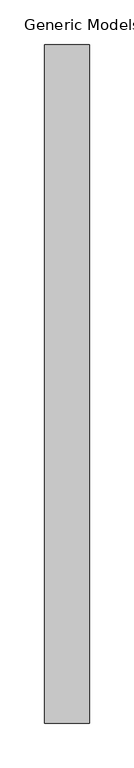
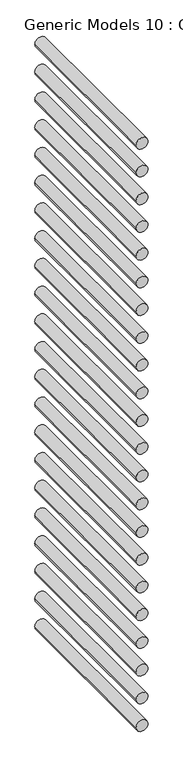
"""IFC4 building model written with IfcOpenShell, lengths in millimetres: proxy geometry, Generic Models 10 : Generic Models 10."""

from ifc_helpers import new_model, si_unit, point, frame, frame_2d, origin, place, context, project, spatial, circle_curve, trimmed, segment, composite_curve, outline, extrude, source, transform, mapped, element, save


def generic_models_10_generic_models_10_d23db068(model_context):
    return source(origin(), model_context, "Body", "SweptSolid", [
        extrude(outline(composite_curve([segment(trimmed(circle_curve(frame_2d((7417.9592795, -4880.4966301)), 25.4), [point((7417.9592795, -4905.8966301))], [point((7417.9592795, -4855.0966301))], False, "CARTESIAN"), True, "CONTINUOUS"), segment(trimmed(circle_curve(frame_2d((7417.9592795, -4880.4966301)), 25.4), [point((7417.9592795, -4855.0966301))], [point((7417.9592795, -4905.8966301))], False, "CARTESIAN"), True, "CONTINUOUS")], self_intersect=False)), frame((0.0, -2396.7968048, 0.0), z_axis=(0.0, 1.0, 0.0), x_axis=(0.0, 0.0, 1.0)), (0.0, 0.0, 1.0), 762.0),
        extrude(outline(composite_curve([segment(trimmed(circle_curve(frame_2d((7290.9592795, -4880.4966301)), 25.4), [point((7290.9592795, -4905.8966301))], [point((7290.9592795, -4855.0966301))], False, "CARTESIAN"), True, "CONTINUOUS"), segment(trimmed(circle_curve(frame_2d((7290.9592795, -4880.4966301)), 25.4), [point((7290.9592795, -4855.0966301))], [point((7290.9592795, -4905.8966301))], False, "CARTESIAN"), True, "CONTINUOUS")], self_intersect=False)), frame((0.0, -2396.7968048, 0.0), z_axis=(0.0, 1.0, 0.0), x_axis=(0.0, 0.0, 1.0)), (0.0, 0.0, 1.0), 762.0),
        extrude(outline(composite_curve([segment(trimmed(circle_curve(frame_2d((7163.9592795, -4880.4966301)), 25.4), [point((7163.9592795, -4905.8966301))], [point((7163.9592795, -4855.0966301))], False, "CARTESIAN"), True, "CONTINUOUS"), segment(trimmed(circle_curve(frame_2d((7163.9592795, -4880.4966301)), 25.4), [point((7163.9592795, -4855.0966301))], [point((7163.9592795, -4905.8966301))], False, "CARTESIAN"), True, "CONTINUOUS")], self_intersect=False)), frame((0.0, -2396.7968048, 0.0), z_axis=(0.0, 1.0, 0.0), x_axis=(0.0, 0.0, 1.0)), (0.0, 0.0, 1.0), 762.0),
        extrude(outline(composite_curve([segment(trimmed(circle_curve(frame_2d((7036.9592795, -4880.4966301)), 25.4), [point((7036.9592795, -4905.8966301))], [point((7036.9592795, -4855.0966301))], False, "CARTESIAN"), True, "CONTINUOUS"), segment(trimmed(circle_curve(frame_2d((7036.9592795, -4880.4966301)), 25.4), [point((7036.9592795, -4855.0966301))], [point((7036.9592795, -4905.8966301))], False, "CARTESIAN"), True, "CONTINUOUS")], self_intersect=False)), frame((0.0, -2396.7968048, 0.0), z_axis=(0.0, 1.0, 0.0), x_axis=(0.0, 0.0, 1.0)), (0.0, 0.0, 1.0), 762.0),
        extrude(outline(composite_curve([segment(trimmed(circle_curve(frame_2d((6909.9592795, -4880.4966301)), 25.4), [point((6909.9592795, -4905.8966301))], [point((6909.9592795, -4855.0966301))], False, "CARTESIAN"), True, "CONTINUOUS"), segment(trimmed(circle_curve(frame_2d((6909.9592795, -4880.4966301)), 25.4), [point((6909.9592795, -4855.0966301))], [point((6909.9592795, -4905.8966301))], False, "CARTESIAN"), True, "CONTINUOUS")], self_intersect=False)), frame((0.0, -2396.7968048, 0.0), z_axis=(0.0, 1.0, 0.0), x_axis=(0.0, 0.0, 1.0)), (0.0, 0.0, 1.0), 762.0),
        extrude(outline(composite_curve([segment(trimmed(circle_curve(frame_2d((6782.9592795, -4880.4966301)), 25.4), [point((6782.9592795, -4905.8966301))], [point((6782.9592795, -4855.0966301))], False, "CARTESIAN"), True, "CONTINUOUS"), segment(trimmed(circle_curve(frame_2d((6782.9592795, -4880.4966301)), 25.4), [point((6782.9592795, -4855.0966301))], [point((6782.9592795, -4905.8966301))], False, "CARTESIAN"), True, "CONTINUOUS")], self_intersect=False)), frame((0.0, -2396.7968048, 0.0), z_axis=(0.0, 1.0, 0.0), x_axis=(0.0, 0.0, 1.0)), (0.0, 0.0, 1.0), 762.0),
        extrude(outline(composite_curve([segment(trimmed(circle_curve(frame_2d((6655.9592795, -4880.4966301)), 25.4), [point((6655.9592795, -4905.8966301))], [point((6655.9592795, -4855.0966301))], False, "CARTESIAN"), True, "CONTINUOUS"), segment(trimmed(circle_curve(frame_2d((6655.9592795, -4880.4966301)), 25.4), [point((6655.9592795, -4855.0966301))], [point((6655.9592795, -4905.8966301))], False, "CARTESIAN"), True, "CONTINUOUS")], self_intersect=False)), frame((0.0, -2396.7968048, 0.0), z_axis=(0.0, 1.0, 0.0), x_axis=(0.0, 0.0, 1.0)), (0.0, 0.0, 1.0), 762.0),
        extrude(outline(composite_curve([segment(trimmed(circle_curve(frame_2d((6528.9592795, -4880.4966301)), 25.4), [point((6528.9592795, -4905.8966301))], [point((6528.9592795, -4855.0966301))], False, "CARTESIAN"), True, "CONTINUOUS"), segment(trimmed(circle_curve(frame_2d((6528.9592795, -4880.4966301)), 25.4), [point((6528.9592795, -4855.0966301))], [point((6528.9592795, -4905.8966301))], False, "CARTESIAN"), True, "CONTINUOUS")], self_intersect=False)), frame((0.0, -2396.7968048, 0.0), z_axis=(0.0, 1.0, 0.0), x_axis=(0.0, 0.0, 1.0)), (0.0, 0.0, 1.0), 762.0),
        extrude(outline(composite_curve([segment(trimmed(circle_curve(frame_2d((6401.9592795, -4880.4966301)), 25.4), [point((6401.9592795, -4905.8966301))], [point((6401.9592795, -4855.0966301))], False, "CARTESIAN"), True, "CONTINUOUS"), segment(trimmed(circle_curve(frame_2d((6401.9592795, -4880.4966301)), 25.4), [point((6401.9592795, -4855.0966301))], [point((6401.9592795, -4905.8966301))], False, "CARTESIAN"), True, "CONTINUOUS")], self_intersect=False)), frame((0.0, -2396.7968048, 0.0), z_axis=(0.0, 1.0, 0.0), x_axis=(0.0, 0.0, 1.0)), (0.0, 0.0, 1.0), 762.0),
        extrude(outline(composite_curve([segment(trimmed(circle_curve(frame_2d((6274.9592795, -4880.4966301)), 25.4), [point((6274.9592795, -4905.8966301))], [point((6274.9592795, -4855.0966301))], False, "CARTESIAN"), True, "CONTINUOUS"), segment(trimmed(circle_curve(frame_2d((6274.9592795, -4880.4966301)), 25.4), [point((6274.9592795, -4855.0966301))], [point((6274.9592795, -4905.8966301))], False, "CARTESIAN"), True, "CONTINUOUS")], self_intersect=False)), frame((0.0, -2396.7968048, 0.0), z_axis=(0.0, 1.0, 0.0), x_axis=(0.0, 0.0, 1.0)), (0.0, 0.0, 1.0), 762.0),
        extrude(outline(composite_curve([segment(trimmed(circle_curve(frame_2d((6147.9592795, -4880.4966301)), 25.4), [point((6147.9592795, -4905.8966301))], [point((6147.9592795, -4855.0966301))], False, "CARTESIAN"), True, "CONTINUOUS"), segment(trimmed(circle_curve(frame_2d((6147.9592795, -4880.4966301)), 25.4), [point((6147.9592795, -4855.0966301))], [point((6147.9592795, -4905.8966301))], False, "CARTESIAN"), True, "CONTINUOUS")], self_intersect=False)), frame((0.0, -2396.7968048, 0.0), z_axis=(0.0, 1.0, 0.0), x_axis=(0.0, 0.0, 1.0)), (0.0, 0.0, 1.0), 762.0),
        extrude(outline(composite_curve([segment(trimmed(circle_curve(frame_2d((6020.9592795, -4880.4966301)), 25.4), [point((6020.9592795, -4905.8966301))], [point((6020.9592795, -4855.0966301))], False, "CARTESIAN"), True, "CONTINUOUS"), segment(trimmed(circle_curve(frame_2d((6020.9592795, -4880.4966301)), 25.4), [point((6020.9592795, -4855.0966301))], [point((6020.9592795, -4905.8966301))], False, "CARTESIAN"), True, "CONTINUOUS")], self_intersect=False)), frame((0.0, -2396.7968048, 0.0), z_axis=(0.0, 1.0, 0.0), x_axis=(0.0, 0.0, 1.0)), (0.0, 0.0, 1.0), 762.0),
        extrude(outline(composite_curve([segment(trimmed(circle_curve(frame_2d((5893.9592795, -4880.4966301)), 25.4), [point((5893.9592795, -4905.8966301))], [point((5893.9592795, -4855.0966301))], False, "CARTESIAN"), True, "CONTINUOUS"), segment(trimmed(circle_curve(frame_2d((5893.9592795, -4880.4966301)), 25.4), [point((5893.9592795, -4855.0966301))], [point((5893.9592795, -4905.8966301))], False, "CARTESIAN"), True, "CONTINUOUS")], self_intersect=False)), frame((0.0, -2396.7968048, 0.0), z_axis=(0.0, 1.0, 0.0), x_axis=(0.0, 0.0, 1.0)), (0.0, 0.0, 1.0), 762.0),
        extrude(outline(composite_curve([segment(trimmed(circle_curve(frame_2d((5766.9592795, -4880.4966301)), 25.4), [point((5766.9592795, -4905.8966301))], [point((5766.9592795, -4855.0966301))], False, "CARTESIAN"), True, "CONTINUOUS"), segment(trimmed(circle_curve(frame_2d((5766.9592795, -4880.4966301)), 25.4), [point((5766.9592795, -4855.0966301))], [point((5766.9592795, -4905.8966301))], False, "CARTESIAN"), True, "CONTINUOUS")], self_intersect=False)), frame((0.0, -2396.7968048, 0.0), z_axis=(0.0, 1.0, 0.0), x_axis=(0.0, 0.0, 1.0)), (0.0, 0.0, 1.0), 762.0),
        extrude(outline(composite_curve([segment(trimmed(circle_curve(frame_2d((5639.9592795, -4880.4966301)), 25.4), [point((5639.9592795, -4905.8966301))], [point((5639.9592795, -4855.0966301))], False, "CARTESIAN"), True, "CONTINUOUS"), segment(trimmed(circle_curve(frame_2d((5639.9592795, -4880.4966301)), 25.4), [point((5639.9592795, -4855.0966301))], [point((5639.9592795, -4905.8966301))], False, "CARTESIAN"), True, "CONTINUOUS")], self_intersect=False)), frame((0.0, -2396.7968048, 0.0), z_axis=(0.0, 1.0, 0.0), x_axis=(0.0, 0.0, 1.0)), (0.0, 0.0, 1.0), 762.0),
        extrude(outline(composite_curve([segment(trimmed(circle_curve(frame_2d((5512.9592795, -4880.4966301)), 25.4), [point((5512.9592795, -4905.8966301))], [point((5512.9592795, -4855.0966301))], False, "CARTESIAN"), True, "CONTINUOUS"), segment(trimmed(circle_curve(frame_2d((5512.9592795, -4880.4966301)), 25.4), [point((5512.9592795, -4855.0966301))], [point((5512.9592795, -4905.8966301))], False, "CARTESIAN"), True, "CONTINUOUS")], self_intersect=False)), frame((0.0, -2396.7968048, 0.0), z_axis=(0.0, 1.0, 0.0), x_axis=(0.0, 0.0, 1.0)), (0.0, 0.0, 1.0), 762.0),
        extrude(outline(composite_curve([segment(trimmed(circle_curve(frame_2d((5385.9592795, -4880.4966301)), 25.4), [point((5385.9592795, -4905.8966301))], [point((5385.9592795, -4855.0966301))], False, "CARTESIAN"), True, "CONTINUOUS"), segment(trimmed(circle_curve(frame_2d((5385.9592795, -4880.4966301)), 25.4), [point((5385.9592795, -4855.0966301))], [point((5385.9592795, -4905.8966301))], False, "CARTESIAN"), True, "CONTINUOUS")], self_intersect=False)), frame((0.0, -2396.7968048, 0.0), z_axis=(0.0, 1.0, 0.0), x_axis=(0.0, 0.0, 1.0)), (0.0, 0.0, 1.0), 762.0),
        extrude(outline(composite_curve([segment(trimmed(circle_curve(frame_2d((5258.9592795, -4880.4966301)), 25.4), [point((5258.9592795, -4905.8966301))], [point((5258.9592795, -4855.0966301))], False, "CARTESIAN"), True, "CONTINUOUS"), segment(trimmed(circle_curve(frame_2d((5258.9592795, -4880.4966301)), 25.4), [point((5258.9592795, -4855.0966301))], [point((5258.9592795, -4905.8966301))], False, "CARTESIAN"), True, "CONTINUOUS")], self_intersect=False)), frame((0.0, -2396.7968048, 0.0), z_axis=(0.0, 1.0, 0.0), x_axis=(0.0, 0.0, 1.0)), (0.0, 0.0, 1.0), 762.0),
        extrude(outline(composite_curve([segment(trimmed(circle_curve(frame_2d((5131.9592795, -4880.4966301)), 25.4), [point((5131.9592795, -4905.8966301))], [point((5131.9592795, -4855.0966301))], False, "CARTESIAN"), True, "CONTINUOUS"), segment(trimmed(circle_curve(frame_2d((5131.9592795, -4880.4966301)), 25.4), [point((5131.9592795, -4855.0966301))], [point((5131.9592795, -4905.8966301))], False, "CARTESIAN"), True, "CONTINUOUS")], self_intersect=False)), frame((0.0, -2396.7968048, 0.0), z_axis=(0.0, 1.0, 0.0), x_axis=(0.0, 0.0, 1.0)), (0.0, 0.0, 1.0), 762.0),
        extrude(outline(composite_curve([segment(trimmed(circle_curve(frame_2d((5004.9592795, -4880.4966301)), 25.4), [point((5004.9592795, -4905.8966301))], [point((5004.9592795, -4855.0966301))], False, "CARTESIAN"), True, "CONTINUOUS"), segment(trimmed(circle_curve(frame_2d((5004.9592795, -4880.4966301)), 25.4), [point((5004.9592795, -4855.0966301))], [point((5004.9592795, -4905.8966301))], False, "CARTESIAN"), True, "CONTINUOUS")], self_intersect=False)), frame((0.0, -2396.7968048, 0.0), z_axis=(0.0, 1.0, 0.0), x_axis=(0.0, 0.0, 1.0)), (0.0, 0.0, 1.0), 762.0),
        extrude(outline(composite_curve([segment(trimmed(circle_curve(frame_2d((4877.9592795, -4880.4966301)), 25.4), [point((4877.9592795, -4905.8966301))], [point((4877.9592795, -4855.0966301))], False, "CARTESIAN"), True, "CONTINUOUS"), segment(trimmed(circle_curve(frame_2d((4877.9592795, -4880.4966301)), 25.4), [point((4877.9592795, -4855.0966301))], [point((4877.9592795, -4905.8966301))], False, "CARTESIAN"), True, "CONTINUOUS")], self_intersect=False)), frame((0.0, -2396.7968048, 0.0), z_axis=(0.0, 1.0, 0.0), x_axis=(0.0, 0.0, 1.0)), (0.0, 0.0, 1.0), 762.0),
        extrude(outline(composite_curve([segment(trimmed(circle_curve(frame_2d((4750.9592795, -4880.4966301)), 25.4), [point((4750.9592795, -4905.8966301))], [point((4750.9592795, -4855.0966301))], False, "CARTESIAN"), True, "CONTINUOUS"), segment(trimmed(circle_curve(frame_2d((4750.9592795, -4880.4966301)), 25.4), [point((4750.9592795, -4855.0966301))], [point((4750.9592795, -4905.8966301))], False, "CARTESIAN"), True, "CONTINUOUS")], self_intersect=False)), frame((0.0, -2396.7968048, 0.0), z_axis=(0.0, 1.0, 0.0), x_axis=(0.0, 0.0, 1.0)), (0.0, 0.0, 1.0), 762.0),
    ])


if __name__ == "__main__":
    model = new_model("IFC4")
    model_context = context("Model", 3, world=origin())
    ifc_project = project(units=[si_unit("LENGTHUNIT", "METRE", prefix="MILLI")], contexts=[model_context])
    site = spatial("IfcSite", under=ifc_project)
    building = spatial("IfcBuilding", under=site)
    placement = place(None, origin())
    generic_models_10_generic_models_10_shape = generic_models_10_generic_models_10_d23db068(model_context)
    element("IfcBuildingElementProxy", 1, Name="Generic Models 10 : Generic Models 10", ObjectType="Generic Models 10 : Generic Models 10", at=placement, inside=building, context=model_context, shape_type="MappedRepresentation", body=[
        mapped(generic_models_10_generic_models_10_shape, transform((0.0, 0.0, 0.0), x_axis=(1.0, 0.0, 0.0), y_axis=(0.0, 1.0, 0.0), z_axis=(0.0, 0.0, 1.0))),
    ])
    save(model, "model.ifc")
